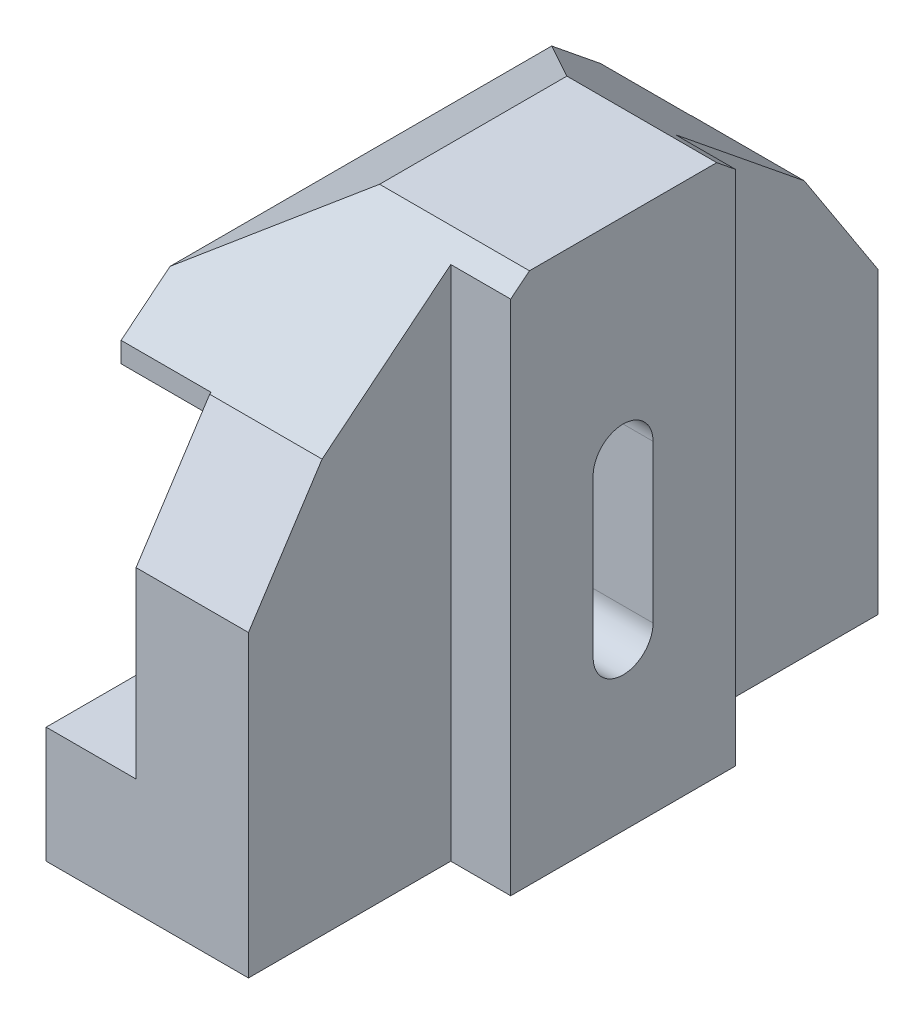
ISO-10303-21;
HEADER;
FILE_DESCRIPTION(('STEP AP214'),'2;1');
FILE_NAME('part.step','',(''),(''),'','','');
FILE_SCHEMA(('AUTOMOTIVE_DESIGN { 1 0 10303 214 1 1 1 1 }'));
ENDSEC;
DATA;
#1=APPLICATION_CONTEXT('core data for automotive mechanical design processes');
#2=APPLICATION_PROTOCOL_DEFINITION('international standard','automotive_design',2000,#1);
#3=PRODUCT_CONTEXT('',#1,'mechanical');
#4=PRODUCT('Part','Part','',(#3));
#5=PRODUCT_RELATED_PRODUCT_CATEGORY('part','',(#4));
#6=PRODUCT_DEFINITION_FORMATION('','',#4);
#7=PRODUCT_DEFINITION_CONTEXT('part definition',#1,'design');
#8=PRODUCT_DEFINITION('design','',#6,#7);
#9=PRODUCT_DEFINITION_SHAPE('','',#8);
#10=(LENGTH_UNIT() NAMED_UNIT(*) SI_UNIT(.MILLI.,.METRE.));
#11=(NAMED_UNIT(*) PLANE_ANGLE_UNIT() SI_UNIT($,.RADIAN.));
#12=(NAMED_UNIT(*) SI_UNIT($,.STERADIAN.) SOLID_ANGLE_UNIT());
#13=UNCERTAINTY_MEASURE_WITH_UNIT(LENGTH_MEASURE(1.E-05),#10,'distance_accuracy_value','');
#14=(GEOMETRIC_REPRESENTATION_CONTEXT(3) GLOBAL_UNCERTAINTY_ASSIGNED_CONTEXT((#13)) GLOBAL_UNIT_ASSIGNED_CONTEXT((#10,
#11,#12)) REPRESENTATION_CONTEXT('',''));
#15=CARTESIAN_POINT('',(0.,0.,0.));
#16=DIRECTION('',(0.,0.,1.));
#17=DIRECTION('',(1.,0.,0.));
#18=AXIS2_PLACEMENT_3D('',#15,#16,#17);
#19=CARTESIAN_POINT('',(27.,0.,84.));
#20=DIRECTION('',(-1.,0.,0.));
#21=DIRECTION('',(0.,0.,1.));
#22=AXIS2_PLACEMENT_3D('',#19,#20,#21);
#23=PLANE('',#22);
#24=DIRECTION('',(0.,-1.,0.));
#25=VECTOR('',#24,1.);
#26=CARTESIAN_POINT('',(27.,71.,57.));
#27=LINE('',#26,#25);
#28=CARTESIAN_POINT('',(27.,68.9755399170125,57.));
#29=VERTEX_POINT('',#28);
#30=CARTESIAN_POINT('',(27.,0.,57.));
#31=VERTEX_POINT('',#30);
#32=EDGE_CURVE('E276',#29,#31,#27,.T.);
#33=ORIENTED_EDGE('',*,*,#32,.F.);
#34=DIRECTION('',(0.,-0.629320391049835,0.777145961456973));
#35=VECTOR('',#34,1.);
#36=CARTESIAN_POINT('',(27.,28.453187913207,107.040937265612));
#37=LINE('',#36,#35);
#38=CARTESIAN_POINT('',(27.,55.0670132063228,74.1756000866226));
#39=VERTEX_POINT('',#38);
#40=EDGE_CURVE('E259',#29,#39,#37,.T.);
#41=ORIENTED_EDGE('',*,*,#40,.T.);
#42=DIRECTION('',(0.,-0.838670567945423,0.544639035015028));
#43=VECTOR('',#42,1.);
#44=CARTESIAN_POINT('',(27.,11.8471025978211,102.242938213101));
#45=LINE('',#44,#43);
#46=CARTESIAN_POINT('',(27.,39.93876398921,84.));
#47=VERTEX_POINT('',#46);
#48=EDGE_CURVE('E275',#39,#47,#45,.T.);
#49=ORIENTED_EDGE('',*,*,#48,.T.);
#50=DIRECTION('',(0.,1.,0.));
#51=VECTOR('',#50,1.);
#52=CARTESIAN_POINT('',(27.,0.,84.));
#53=LINE('',#52,#51);
#54=CARTESIAN_POINT('',(27.,0.,84.));
#55=VERTEX_POINT('',#54);
#56=EDGE_CURVE('E316',#55,#47,#53,.T.);
#57=ORIENTED_EDGE('',*,*,#56,.F.);
#58=DIRECTION('',(0.,0.,-1.));
#59=VECTOR('',#58,1.);
#60=CARTESIAN_POINT('',(27.,0.,84.));
#61=LINE('',#60,#59);
#62=EDGE_CURVE('E358',#55,#31,#61,.T.);
#63=ORIENTED_EDGE('',*,*,#62,.T.);
#64=EDGE_LOOP('',(#33,#41,#49,#57,#63));
#65=FACE_BOUND('',#64,.T.);
#66=ADVANCED_FACE('F39',(#65),#23,.F.);
#67=CARTESIAN_POINT('',(15.,71.,84.));
#68=DIRECTION('',(0.573576436351045,-0.819152044288992,0.));
#69=DIRECTION('',(0.819152044288992,0.573576436351045,0.));
#70=AXIS2_PLACEMENT_3D('',#67,#68,#69);
#71=PLANE('',#70);
#72=DIRECTION('',(0.,0.,-1.));
#73=VECTOR('',#72,1.);
#74=CARTESIAN_POINT('',(15.,71.,84.));
#75=LINE('',#74,#73);
#76=CARTESIAN_POINT('',(15.,71.,54.5));
#77=VERTEX_POINT('',#76);
#78=CARTESIAN_POINT('',(15.,71.,29.5));
#79=VERTEX_POINT('',#78);
#80=EDGE_CURVE('E354',#77,#79,#75,.T.);
#81=ORIENTED_EDGE('',*,*,#80,.T.);
#82=DIRECTION('',(-0.66845613754,-0.468058026468054,-0.578003525978809));
#83=VECTOR('',#82,1.);
#84=CARTESIAN_POINT('',(36.0571652430861,85.7443858365364,47.7078001443945));
#85=LINE('',#84,#83);
#86=CARTESIAN_POINT('',(0.,60.4968869268544,16.5297355312063));
#87=VERTEX_POINT('',#86);
#88=EDGE_CURVE('E255',#79,#87,#85,.T.);
#89=ORIENTED_EDGE('',*,*,#88,.T.);
#90=DIRECTION('',(0.,0.,-1.));
#91=VECTOR('',#90,1.);
#92=CARTESIAN_POINT('',(0.,60.4968869268544,84.));
#93=LINE('',#92,#91);
#94=CARTESIAN_POINT('',(0.,60.4968869268544,67.4702644687937));
#95=VERTEX_POINT('',#94);
#96=EDGE_CURVE('E348',#95,#87,#93,.T.);
#97=ORIENTED_EDGE('',*,*,#96,.F.);
#98=DIRECTION('',(0.668456137539999,0.468058026468053,-0.57800352597881));
#99=VECTOR('',#98,1.);
#100=CARTESIAN_POINT('',(3.60208486842126,63.0190939049941,64.3555982432961));
#101=LINE('',#100,#99);
#102=EDGE_CURVE('E266',#95,#77,#101,.T.);
#103=ORIENTED_EDGE('',*,*,#102,.T.);
#104=EDGE_LOOP('',(#81,#89,#97,#103));
#105=FACE_BOUND('',#104,.T.);
#106=ADVANCED_FACE('F400',(#105),#71,.F.);
#107=CARTESIAN_POINT('',(0.,60.4968869268544,84.));
#108=DIRECTION('',(1.,0.,0.));
#109=DIRECTION('',(0.,1.,0.));
#110=AXIS2_PLACEMENT_3D('',#107,#108,#109);
#111=PLANE('',#110);
#112=ORIENTED_EDGE('',*,*,#96,.T.);
#113=DIRECTION('',(0.,-0.629320391049836,-0.777145961456972));
#114=VECTOR('',#113,1.);
#115=CARTESIAN_POINT('',(0.,93.4948255823673,57.2787961484174));
#116=LINE('',#115,#114);
#117=CARTESIAN_POINT('',(0.,55.2092113526974,10.));
#118=VERTEX_POINT('',#117);
#119=EDGE_CURVE('E248',#87,#118,#116,.T.);
#120=ORIENTED_EDGE('',*,*,#119,.T.);
#121=DIRECTION('',(0.,-1.,0.));
#122=VECTOR('',#121,1.);
#123=CARTESIAN_POINT('',(0.,99.4968869268544,10.));
#124=LINE('',#123,#122);
#125=CARTESIAN_POINT('',(0.,52.4968869268544,10.));
#126=VERTEX_POINT('',#125);
#127=EDGE_CURVE('E296',#118,#126,#124,.T.);
#128=ORIENTED_EDGE('',*,*,#127,.T.);
#129=DIRECTION('',(0.,0.,-1.));
#130=VECTOR('',#129,1.);
#131=CARTESIAN_POINT('',(0.,52.4968869268544,84.));
#132=LINE('',#131,#130);
#133=CARTESIAN_POINT('',(0.,52.4968869268544,74.));
#134=VERTEX_POINT('',#133);
#135=EDGE_CURVE('E349',#134,#126,#132,.T.);
#136=ORIENTED_EDGE('',*,*,#135,.F.);
#137=DIRECTION('',(0.,-1.,0.));
#138=VECTOR('',#137,1.);
#139=CARTESIAN_POINT('',(0.,99.4968869268544,74.));
#140=LINE('',#139,#138);
#141=CARTESIAN_POINT('',(0.,55.2092113526974,74.));
#142=VERTEX_POINT('',#141);
#143=EDGE_CURVE('E299',#142,#134,#140,.T.);
#144=ORIENTED_EDGE('',*,*,#143,.F.);
#145=DIRECTION('',(0.,0.629320391049835,-0.777145961456973));
#146=VECTOR('',#145,1.);
#147=CARTESIAN_POINT('',(0.,52.4126263515475,77.4534948659287));
#148=LINE('',#147,#146);
#149=EDGE_CURVE('E267',#142,#95,#148,.T.);
#150=ORIENTED_EDGE('',*,*,#149,.T.);
#151=EDGE_LOOP('',(#112,#120,#128,#136,#144,#150));
#152=FACE_BOUND('',#151,.T.);
#153=ADVANCED_FACE('F407',(#152),#111,.F.);
#154=CARTESIAN_POINT('',(0.,52.4968869268544,84.));
#155=DIRECTION('',(0.,1.,0.));
#156=DIRECTION('',(0.,0.,1.));
#157=AXIS2_PLACEMENT_3D('',#154,#155,#156);
#158=PLANE('',#157);
#159=DIRECTION('',(1.,0.,0.));
#160=VECTOR('',#159,1.);
#161=CARTESIAN_POINT('',(0.,52.4968869268544,74.));
#162=LINE('',#161,#160);
#163=CARTESIAN_POINT('',(12.,52.4968869268544,74.));
#164=VERTEX_POINT('',#163);
#165=EDGE_CURVE('E307',#134,#164,#162,.T.);
#166=ORIENTED_EDGE('',*,*,#165,.F.);
#167=ORIENTED_EDGE('',*,*,#135,.T.);
#168=DIRECTION('',(-1.,0.,0.));
#169=VECTOR('',#168,1.);
#170=CARTESIAN_POINT('',(0.,52.4968869268544,10.));
#171=LINE('',#170,#169);
#172=CARTESIAN_POINT('',(12.,52.4968869268544,10.));
#173=VERTEX_POINT('',#172);
#174=EDGE_CURVE('E302',#173,#126,#171,.T.);
#175=ORIENTED_EDGE('',*,*,#174,.F.);
#176=DIRECTION('',(0.,0.,-1.));
#177=VECTOR('',#176,1.);
#178=CARTESIAN_POINT('',(12.,52.4968869268544,84.));
#179=LINE('',#178,#177);
#180=EDGE_CURVE('E344',#164,#173,#179,.T.);
#181=ORIENTED_EDGE('',*,*,#180,.F.);
#182=EDGE_LOOP('',(#166,#167,#175,#181));
#183=FACE_BOUND('',#182,.T.);
#184=ADVANCED_FACE('F477',(#183),#158,.F.);
#185=CARTESIAN_POINT('',(0.,0.,84.));
#186=DIRECTION('',(0.,0.,1.));
#187=DIRECTION('',(1.,0.,0.));
#188=AXIS2_PLACEMENT_3D('',#185,#186,#187);
#189=PLANE('',#188);
#190=DIRECTION('',(1.,0.,0.));
#191=VECTOR('',#190,1.);
#192=CARTESIAN_POINT('',(-15.5,39.93876398921,84.));
#193=LINE('',#192,#191);
#194=CARTESIAN_POINT('',(12.,39.93876398921,84.));
#195=VERTEX_POINT('',#194);
#196=EDGE_CURVE('E235',#195,#47,#193,.T.);
#197=ORIENTED_EDGE('',*,*,#196,.F.);
#198=DIRECTION('',(0.,-1.,0.));
#199=VECTOR('',#198,1.);
#200=CARTESIAN_POINT('',(12.,52.4968869268544,84.));
#201=LINE('',#200,#199);
#202=CARTESIAN_POINT('',(12.,15.4968869268544,84.));
#203=VERTEX_POINT('',#202);
#204=EDGE_CURVE('E325',#195,#203,#201,.T.);
#205=ORIENTED_EDGE('',*,*,#204,.T.);
#206=DIRECTION('',(-1.,0.,0.));
#207=VECTOR('',#206,1.);
#208=CARTESIAN_POINT('',(12.,15.4968869268544,84.));
#209=LINE('',#208,#207);
#210=CARTESIAN_POINT('',(0.,15.4968869268544,84.));
#211=VERTEX_POINT('',#210);
#212=EDGE_CURVE('E321',#203,#211,#209,.T.);
#213=ORIENTED_EDGE('',*,*,#212,.T.);
#214=DIRECTION('',(0.,-1.,0.));
#215=VECTOR('',#214,1.);
#216=CARTESIAN_POINT('',(0.,15.4968869268544,84.));
#217=LINE('',#216,#215);
#218=CARTESIAN_POINT('',(0.,0.,84.));
#219=VERTEX_POINT('',#218);
#220=EDGE_CURVE('E312',#211,#219,#217,.T.);
#221=ORIENTED_EDGE('',*,*,#220,.T.);
#222=DIRECTION('',(1.,0.,0.));
#223=VECTOR('',#222,1.);
#224=CARTESIAN_POINT('',(0.,0.,84.));
#225=LINE('',#224,#223);
#226=EDGE_CURVE('E317',#219,#55,#225,.T.);
#227=ORIENTED_EDGE('',*,*,#226,.T.);
#228=ORIENTED_EDGE('',*,*,#56,.T.);
#229=EDGE_LOOP('',(#197,#205,#213,#221,#227,#228));
#230=FACE_BOUND('',#229,.T.);
#231=ADVANCED_FACE('F463',(#230),#189,.T.);
#232=CARTESIAN_POINT('',(0.,0.,0.));
#233=DIRECTION('',(0.,0.,1.));
#234=DIRECTION('',(1.,0.,0.));
#235=AXIS2_PLACEMENT_3D('',#232,#233,#234);
#236=PLANE('',#235);
#237=DIRECTION('',(0.,-1.,0.));
#238=VECTOR('',#237,1.);
#239=CARTESIAN_POINT('',(12.,52.4968869268544,0.));
#240=LINE('',#239,#238);
#241=CARTESIAN_POINT('',(12.,39.93876398921,0.));
#242=VERTEX_POINT('',#241);
#243=CARTESIAN_POINT('',(12.,15.4968869268544,0.));
#244=VERTEX_POINT('',#243);
#245=EDGE_CURVE('E333',#242,#244,#240,.T.);
#246=ORIENTED_EDGE('',*,*,#245,.F.);
#247=DIRECTION('',(1.,0.,0.));
#248=VECTOR('',#247,1.);
#249=CARTESIAN_POINT('',(-15.5,39.93876398921,0.));
#250=LINE('',#249,#248);
#251=CARTESIAN_POINT('',(27.,39.93876398921,0.));
#252=VERTEX_POINT('',#251);
#253=EDGE_CURVE('E225',#242,#252,#250,.T.);
#254=ORIENTED_EDGE('',*,*,#253,.T.);
#255=DIRECTION('',(0.,1.,0.));
#256=VECTOR('',#255,1.);
#257=CARTESIAN_POINT('',(27.,0.,0.));
#258=LINE('',#257,#256);
#259=CARTESIAN_POINT('',(27.,0.,0.));
#260=VERTEX_POINT('',#259);
#261=EDGE_CURVE('E334',#260,#252,#258,.T.);
#262=ORIENTED_EDGE('',*,*,#261,.F.);
#263=DIRECTION('',(1.,0.,0.));
#264=VECTOR('',#263,1.);
#265=CARTESIAN_POINT('',(0.,0.,0.));
#266=LINE('',#265,#264);
#267=CARTESIAN_POINT('',(0.,0.,0.));
#268=VERTEX_POINT('',#267);
#269=EDGE_CURVE('E328',#268,#260,#266,.T.);
#270=ORIENTED_EDGE('',*,*,#269,.F.);
#271=DIRECTION('',(0.,-1.,0.));
#272=VECTOR('',#271,1.);
#273=CARTESIAN_POINT('',(0.,15.4968869268544,0.));
#274=LINE('',#273,#272);
#275=CARTESIAN_POINT('',(0.,15.4968869268544,0.));
#276=VERTEX_POINT('',#275);
#277=EDGE_CURVE('E315',#276,#268,#274,.T.);
#278=ORIENTED_EDGE('',*,*,#277,.F.);
#279=DIRECTION('',(-1.,0.,0.));
#280=VECTOR('',#279,1.);
#281=CARTESIAN_POINT('',(12.,15.4968869268544,0.));
#282=LINE('',#281,#280);
#283=EDGE_CURVE('E320',#244,#276,#282,.T.);
#284=ORIENTED_EDGE('',*,*,#283,.F.);
#285=EDGE_LOOP('',(#246,#254,#262,#270,#278,#284));
#286=FACE_BOUND('',#285,.T.);
#287=ADVANCED_FACE('F424',(#286),#236,.F.);
#288=CARTESIAN_POINT('',(0.,15.4968869268544,84.));
#289=DIRECTION('',(1.,0.,0.));
#290=DIRECTION('',(0.,1.,0.));
#291=AXIS2_PLACEMENT_3D('',#288,#289,#290);
#292=PLANE('',#291);
#293=ORIENTED_EDGE('',*,*,#277,.T.);
#294=DIRECTION('',(0.,0.,-1.));
#295=VECTOR('',#294,1.);
#296=CARTESIAN_POINT('',(0.,0.,84.));
#297=LINE('',#296,#295);
#298=EDGE_CURVE('E360',#219,#268,#297,.T.);
#299=ORIENTED_EDGE('',*,*,#298,.F.);
#300=ORIENTED_EDGE('',*,*,#220,.F.);
#301=DIRECTION('',(0.,0.,-1.));
#302=VECTOR('',#301,1.);
#303=CARTESIAN_POINT('',(0.,15.4968869268544,84.));
#304=LINE('',#303,#302);
#305=EDGE_CURVE('E329',#211,#276,#304,.T.);
#306=ORIENTED_EDGE('',*,*,#305,.T.);
#307=EDGE_LOOP('',(#293,#299,#300,#306));
#308=FACE_BOUND('',#307,.T.);
#309=ADVANCED_FACE('F41',(#308),#292,.F.);
#310=CARTESIAN_POINT('',(0.,0.,84.));
#311=DIRECTION('',(0.,1.,0.));
#312=DIRECTION('',(0.,0.,1.));
#313=AXIS2_PLACEMENT_3D('',#310,#311,#312);
#314=PLANE('',#313);
#315=ORIENTED_EDGE('',*,*,#269,.T.);
#316=CARTESIAN_POINT('',(27.,0.,27.));
#317=VERTEX_POINT('',#316);
#318=EDGE_CURVE('E353',#317,#260,#61,.T.);
#319=ORIENTED_EDGE('',*,*,#318,.F.);
#320=DIRECTION('',(1.,0.,0.));
#321=VECTOR('',#320,1.);
#322=CARTESIAN_POINT('',(27.,0.,27.));
#323=LINE('',#322,#321);
#324=CARTESIAN_POINT('',(35.,0.,27.));
#325=VERTEX_POINT('',#324);
#326=EDGE_CURVE('E286',#317,#325,#323,.T.);
#327=ORIENTED_EDGE('',*,*,#326,.T.);
#328=DIRECTION('',(0.,0.,-1.));
#329=VECTOR('',#328,1.);
#330=CARTESIAN_POINT('',(35.,0.,57.));
#331=LINE('',#330,#329);
#332=CARTESIAN_POINT('',(35.,0.,57.));
#333=VERTEX_POINT('',#332);
#334=EDGE_CURVE('E294',#333,#325,#331,.T.);
#335=ORIENTED_EDGE('',*,*,#334,.F.);
#336=DIRECTION('',(1.,0.,0.));
#337=VECTOR('',#336,1.);
#338=CARTESIAN_POINT('',(27.,0.,57.));
#339=LINE('',#338,#337);
#340=EDGE_CURVE('E284',#31,#333,#339,.T.);
#341=ORIENTED_EDGE('',*,*,#340,.F.);
#342=ORIENTED_EDGE('',*,*,#62,.F.);
#343=ORIENTED_EDGE('',*,*,#226,.F.);
#344=ORIENTED_EDGE('',*,*,#298,.T.);
#345=EDGE_LOOP('',(#315,#319,#327,#335,#341,#342,#343,#344));
#346=FACE_BOUND('',#345,.T.);
#347=ADVANCED_FACE('F415',(#346),#314,.F.);
#348=ORIENTED_EDGE('',*,*,#261,.T.);
#349=DIRECTION('',(0.,0.838670567945423,0.544639035015029));
#350=VECTOR('',#349,1.);
#351=CARTESIAN_POINT('',(27.,50.2160118188104,6.67412277771519));
#352=LINE('',#351,#350);
#353=CARTESIAN_POINT('',(27.,55.0670132063228,9.82439991337739));
#354=VERTEX_POINT('',#353);
#355=EDGE_CURVE('E273',#252,#354,#352,.T.);
#356=ORIENTED_EDGE('',*,*,#355,.T.);
#357=DIRECTION('',(0.,0.629320391049836,0.777145961456972));
#358=VECTOR('',#357,1.);
#359=CARTESIAN_POINT('',(27.,69.5353871440268,27.691353748734));
#360=LINE('',#359,#358);
#361=CARTESIAN_POINT('',(27.,68.9755399170125,27.));
#362=VERTEX_POINT('',#361);
#363=EDGE_CURVE('E241',#354,#362,#360,.T.);
#364=ORIENTED_EDGE('',*,*,#363,.T.);
#365=DIRECTION('',(0.,-1.,0.));
#366=VECTOR('',#365,1.);
#367=CARTESIAN_POINT('',(27.,71.,27.));
#368=LINE('',#367,#366);
#369=EDGE_CURVE('E279',#362,#317,#368,.T.);
#370=ORIENTED_EDGE('',*,*,#369,.T.);
#371=ORIENTED_EDGE('',*,*,#318,.T.);
#372=EDGE_LOOP('',(#348,#356,#364,#370,#371));
#373=FACE_BOUND('',#372,.T.);
#374=ADVANCED_FACE('F402',(#373),#23,.F.);
#375=CARTESIAN_POINT('',(27.,71.,84.));
#376=DIRECTION('',(0.,-1.,0.));
#377=DIRECTION('',(0.,0.,-1.));
#378=AXIS2_PLACEMENT_3D('',#375,#376,#377);
#379=PLANE('',#378);
#380=DIRECTION('',(0.,0.,-1.));
#381=VECTOR('',#380,1.);
#382=CARTESIAN_POINT('',(35.,71.,57.));
#383=LINE('',#382,#381);
#384=CARTESIAN_POINT('',(35.,71.,54.5));
#385=VERTEX_POINT('',#384);
#386=CARTESIAN_POINT('',(35.,71.,29.5));
#387=VERTEX_POINT('',#386);
#388=EDGE_CURVE('E289',#385,#387,#383,.T.);
#389=ORIENTED_EDGE('',*,*,#388,.T.);
#390=DIRECTION('',(1.,0.,0.));
#391=VECTOR('',#390,1.);
#392=CARTESIAN_POINT('',(-15.5,71.,29.5));
#393=LINE('',#392,#391);
#394=EDGE_CURVE('E229',#79,#387,#393,.T.);
#395=ORIENTED_EDGE('',*,*,#394,.F.);
#396=ORIENTED_EDGE('',*,*,#80,.F.);
#397=DIRECTION('',(1.,0.,0.));
#398=VECTOR('',#397,1.);
#399=CARTESIAN_POINT('',(-15.5,71.,54.5));
#400=LINE('',#399,#398);
#401=EDGE_CURVE('E217',#77,#385,#400,.T.);
#402=ORIENTED_EDGE('',*,*,#401,.T.);
#403=EDGE_LOOP('',(#389,#395,#396,#402));
#404=FACE_BOUND('',#403,.T.);
#405=ADVANCED_FACE('F411',(#404),#379,.F.);
#406=CARTESIAN_POINT('',(12.,52.4968869268544,84.));
#407=DIRECTION('',(1.,0.,0.));
#408=DIRECTION('',(0.,1.,0.));
#409=AXIS2_PLACEMENT_3D('',#406,#407,#408);
#410=PLANE('',#409);
#411=DIRECTION('',(0.,-1.,0.));
#412=VECTOR('',#411,1.);
#413=CARTESIAN_POINT('',(12.,43.0355530867048,38.));
#414=LINE('',#413,#412);
#415=CARTESIAN_POINT('',(12.,43.0355530867048,38.));
#416=VERTEX_POINT('',#415);
#417=CARTESIAN_POINT('',(12.,22.0355530867048,38.));
#418=VERTEX_POINT('',#417);
#419=EDGE_CURVE('E207',#416,#418,#414,.T.);
#420=ORIENTED_EDGE('',*,*,#419,.F.);
#421=CARTESIAN_POINT('',(12.,43.0355530867048,42.));
#422=DIRECTION('',(-1.,0.,0.));
#423=DIRECTION('',(0.,-1.,0.));
#424=AXIS2_PLACEMENT_3D('',#421,#422,#423);
#425=CIRCLE('',#424,4.);
#426=CARTESIAN_POINT('',(12.,43.0355530867048,46.));
#427=VERTEX_POINT('',#426);
#428=EDGE_CURVE('E53',#427,#416,#425,.T.);
#429=ORIENTED_EDGE('',*,*,#428,.F.);
#430=DIRECTION('',(0.,1.,0.));
#431=VECTOR('',#430,1.);
#432=CARTESIAN_POINT('',(12.,43.0355530867048,46.));
#433=LINE('',#432,#431);
#434=CARTESIAN_POINT('',(12.,22.0355530867048,46.));
#435=VERTEX_POINT('',#434);
#436=EDGE_CURVE('E214',#435,#427,#433,.T.);
#437=ORIENTED_EDGE('',*,*,#436,.F.);
#438=CARTESIAN_POINT('',(12.,22.0355530867048,42.));
#439=DIRECTION('',(-1.,0.,0.));
#440=DIRECTION('',(0.,-1.,0.));
#441=AXIS2_PLACEMENT_3D('',#438,#439,#440);
#442=CIRCLE('',#441,3.99999999999999);
#443=EDGE_CURVE('E196',#418,#435,#442,.T.);
#444=ORIENTED_EDGE('',*,*,#443,.F.);
#445=EDGE_LOOP('',(#420,#429,#437,#444));
#446=FACE_BOUND('',#445,.T.);
#447=DIRECTION('',(0.,-0.629320391049836,-0.777145961456972));
#448=VECTOR('',#447,1.);
#449=CARTESIAN_POINT('',(12.,90.3264723456383,53.3662057454822));
#450=LINE('',#449,#448);
#451=CARTESIAN_POINT('',(12.,55.2092113526974,10.));
#452=VERTEX_POINT('',#451);
#453=CARTESIAN_POINT('',(12.,55.0670132063228,9.82439991337739));
#454=VERTEX_POINT('',#453);
#455=EDGE_CURVE('E246',#452,#454,#450,.T.);
#456=ORIENTED_EDGE('',*,*,#455,.T.);
#457=DIRECTION('',(0.,-0.838670567945423,-0.544639035015029));
#458=VECTOR('',#457,1.);
#459=CARTESIAN_POINT('',(12.,87.1406590625168,30.6532690739178));
#460=LINE('',#459,#458);
#461=EDGE_CURVE('E369',#454,#242,#460,.T.);
#462=ORIENTED_EDGE('',*,*,#461,.T.);
#463=ORIENTED_EDGE('',*,*,#245,.T.);
#464=DIRECTION('',(0.,0.,-1.));
#465=VECTOR('',#464,1.);
#466=CARTESIAN_POINT('',(12.,15.4968869268544,84.));
#467=LINE('',#466,#465);
#468=EDGE_CURVE('E338',#203,#244,#467,.T.);
#469=ORIENTED_EDGE('',*,*,#468,.F.);
#470=ORIENTED_EDGE('',*,*,#204,.F.);
#471=DIRECTION('',(0.,0.838670567945423,-0.544639035015028));
#472=VECTOR('',#471,1.);
#473=CARTESIAN_POINT('',(12.,48.7717498415275,78.2637919168988));
#474=LINE('',#473,#472);
#475=CARTESIAN_POINT('',(12.,55.0670132063228,74.1756000866226));
#476=VERTEX_POINT('',#475);
#477=EDGE_CURVE('E370',#195,#476,#474,.T.);
#478=ORIENTED_EDGE('',*,*,#477,.T.);
#479=DIRECTION('',(0.,0.629320391049835,-0.777145961456973));
#480=VECTOR('',#479,1.);
#481=CARTESIAN_POINT('',(12.,49.2442731148185,81.3660852688639));
#482=LINE('',#481,#480);
#483=CARTESIAN_POINT('',(12.,55.2092113526974,74.));
#484=VERTEX_POINT('',#483);
#485=EDGE_CURVE('E265',#476,#484,#482,.T.);
#486=ORIENTED_EDGE('',*,*,#485,.T.);
#487=DIRECTION('',(0.,-1.,0.));
#488=VECTOR('',#487,1.);
#489=CARTESIAN_POINT('',(12.,99.4968869268544,74.));
#490=LINE('',#489,#488);
#491=EDGE_CURVE('E301',#484,#164,#490,.T.);
#492=ORIENTED_EDGE('',*,*,#491,.T.);
#493=ORIENTED_EDGE('',*,*,#180,.T.);
#494=DIRECTION('',(0.,-1.,0.));
#495=VECTOR('',#494,1.);
#496=CARTESIAN_POINT('',(12.,99.4968869268544,10.));
#497=LINE('',#496,#495);
#498=EDGE_CURVE('E305',#452,#173,#497,.T.);
#499=ORIENTED_EDGE('',*,*,#498,.F.);
#500=EDGE_LOOP('',(#456,#462,#463,#469,#470,#478,#486,#492,#493,#499));
#501=FACE_BOUND('',#500,.T.);
#502=ADVANCED_FACE('F208',(#446,#501),#410,.F.);
#503=CARTESIAN_POINT('',(12.,15.4968869268544,84.));
#504=DIRECTION('',(0.,-1.,0.));
#505=DIRECTION('',(1.,0.,0.));
#506=AXIS2_PLACEMENT_3D('',#503,#504,#505);
#507=PLANE('',#506);
#508=ORIENTED_EDGE('',*,*,#283,.T.);
#509=ORIENTED_EDGE('',*,*,#305,.F.);
#510=ORIENTED_EDGE('',*,*,#212,.F.);
#511=ORIENTED_EDGE('',*,*,#468,.T.);
#512=EDGE_LOOP('',(#508,#509,#510,#511));
#513=FACE_BOUND('',#512,.T.);
#514=ADVANCED_FACE('F457',(#513),#507,.F.);
#515=CARTESIAN_POINT('',(0.,99.4968869268544,10.));
#516=DIRECTION('',(0.,0.,-1.));
#517=DIRECTION('',(-1.,0.,0.));
#518=AXIS2_PLACEMENT_3D('',#515,#516,#517);
#519=PLANE('',#518);
#520=DIRECTION('',(-1.,0.,0.));
#521=VECTOR('',#520,1.);
#522=CARTESIAN_POINT('',(0.,55.2092113526974,10.));
#523=LINE('',#522,#521);
#524=EDGE_CURVE('E242',#452,#118,#523,.T.);
#525=ORIENTED_EDGE('',*,*,#524,.F.);
#526=ORIENTED_EDGE('',*,*,#498,.T.);
#527=ORIENTED_EDGE('',*,*,#174,.T.);
#528=ORIENTED_EDGE('',*,*,#127,.F.);
#529=EDGE_LOOP('',(#525,#526,#527,#528));
#530=FACE_BOUND('',#529,.T.);
#531=ADVANCED_FACE('F438',(#530),#519,.T.);
#532=CARTESIAN_POINT('',(0.,99.4968869268544,74.));
#533=DIRECTION('',(0.,0.,1.));
#534=DIRECTION('',(1.,0.,0.));
#535=AXIS2_PLACEMENT_3D('',#532,#533,#534);
#536=PLANE('',#535);
#537=DIRECTION('',(1.,0.,0.));
#538=VECTOR('',#537,1.);
#539=CARTESIAN_POINT('',(0.,55.2092113526974,74.));
#540=LINE('',#539,#538);
#541=EDGE_CURVE('E264',#142,#484,#540,.T.);
#542=ORIENTED_EDGE('',*,*,#541,.F.);
#543=ORIENTED_EDGE('',*,*,#143,.T.);
#544=ORIENTED_EDGE('',*,*,#165,.T.);
#545=ORIENTED_EDGE('',*,*,#491,.F.);
#546=EDGE_LOOP('',(#542,#543,#544,#545));
#547=FACE_BOUND('',#546,.T.);
#548=ADVANCED_FACE('F479',(#547),#536,.T.);
#549=CARTESIAN_POINT('',(35.,71.,57.));
#550=DIRECTION('',(-1.,0.,0.));
#551=DIRECTION('',(0.,-1.,0.));
#552=AXIS2_PLACEMENT_3D('',#549,#550,#551);
#553=PLANE('',#552);
#554=DIRECTION('',(0.,1.,0.));
#555=VECTOR('',#554,1.);
#556=CARTESIAN_POINT('',(35.,71.,46.));
#557=LINE('',#556,#555);
#558=CARTESIAN_POINT('',(35.,22.0355530867048,46.));
#559=VERTEX_POINT('',#558);
#560=CARTESIAN_POINT('',(35.,43.0355530867048,46.));
#561=VERTEX_POINT('',#560);
#562=EDGE_CURVE('E50',#559,#561,#557,.T.);
#563=ORIENTED_EDGE('',*,*,#562,.T.);
#564=CARTESIAN_POINT('',(35.,43.0355530867048,42.));
#565=DIRECTION('',(-1.,0.,0.));
#566=DIRECTION('',(0.,-1.,0.));
#567=AXIS2_PLACEMENT_3D('',#564,#565,#566);
#568=CIRCLE('',#567,4.);
#569=CARTESIAN_POINT('',(35.,43.0355530867048,38.));
#570=VERTEX_POINT('',#569);
#571=EDGE_CURVE('E11',#561,#570,#568,.T.);
#572=ORIENTED_EDGE('',*,*,#571,.T.);
#573=DIRECTION('',(0.,-1.,0.));
#574=VECTOR('',#573,1.);
#575=CARTESIAN_POINT('',(35.,71.,38.));
#576=LINE('',#575,#574);
#577=CARTESIAN_POINT('',(35.,22.0355530867048,38.));
#578=VERTEX_POINT('',#577);
#579=EDGE_CURVE('E373',#570,#578,#576,.T.);
#580=ORIENTED_EDGE('',*,*,#579,.T.);
#581=CARTESIAN_POINT('',(35.,22.0355530867048,42.));
#582=DIRECTION('',(-1.,0.,0.));
#583=DIRECTION('',(0.,-1.,0.));
#584=AXIS2_PLACEMENT_3D('',#581,#582,#583);
#585=CIRCLE('',#584,3.99999999999999);
#586=EDGE_CURVE('E197',#578,#559,#585,.T.);
#587=ORIENTED_EDGE('',*,*,#586,.T.);
#588=EDGE_LOOP('',(#563,#572,#580,#587));
#589=FACE_BOUND('',#588,.T.);
#590=DIRECTION('',(0.,1.,0.));
#591=VECTOR('',#590,1.);
#592=CARTESIAN_POINT('',(35.,71.,27.));
#593=LINE('',#592,#591);
#594=CARTESIAN_POINT('',(35.,68.9755399170125,27.));
#595=VERTEX_POINT('',#594);
#596=EDGE_CURVE('E281',#325,#595,#593,.T.);
#597=ORIENTED_EDGE('',*,*,#596,.T.);
#598=DIRECTION('',(0.,0.629320391049836,0.777145961456972));
#599=VECTOR('',#598,1.);
#600=CARTESIAN_POINT('',(35.,84.4495295100898,46.1087857487442));
#601=LINE('',#600,#599);
#602=EDGE_CURVE('E228',#595,#387,#601,.T.);
#603=ORIENTED_EDGE('',*,*,#602,.T.);
#604=ORIENTED_EDGE('',*,*,#388,.F.);
#605=DIRECTION('',(0.,-0.629320391049835,0.777145961456973));
#606=VECTOR('',#605,1.);
#607=CARTESIAN_POINT('',(35.,69.7773154990827,56.0098896135222));
#608=LINE('',#607,#606);
#609=CARTESIAN_POINT('',(35.,68.9755399170125,57.));
#610=VERTEX_POINT('',#609);
#611=EDGE_CURVE('E253',#385,#610,#608,.T.);
#612=ORIENTED_EDGE('',*,*,#611,.T.);
#613=DIRECTION('',(0.,1.,0.));
#614=VECTOR('',#613,1.);
#615=CARTESIAN_POINT('',(35.,71.,57.));
#616=LINE('',#615,#614);
#617=EDGE_CURVE('E283',#333,#610,#616,.T.);
#618=ORIENTED_EDGE('',*,*,#617,.F.);
#619=ORIENTED_EDGE('',*,*,#334,.T.);
#620=EDGE_LOOP('',(#597,#603,#604,#612,#618,#619));
#621=FACE_BOUND('',#620,.T.);
#622=ADVANCED_FACE('F380',(#589,#621),#553,.F.);
#623=CARTESIAN_POINT('',(0.,0.,57.));
#624=DIRECTION('',(0.,0.,1.));
#625=DIRECTION('',(1.,0.,0.));
#626=AXIS2_PLACEMENT_3D('',#623,#624,#625);
#627=PLANE('',#626);
#628=DIRECTION('',(1.,0.,0.));
#629=VECTOR('',#628,1.);
#630=CARTESIAN_POINT('',(0.,68.9755399170125,57.));
#631=LINE('',#630,#629);
#632=EDGE_CURVE('E362',#29,#610,#631,.T.);
#633=ORIENTED_EDGE('',*,*,#632,.F.);
#634=ORIENTED_EDGE('',*,*,#32,.T.);
#635=ORIENTED_EDGE('',*,*,#340,.T.);
#636=ORIENTED_EDGE('',*,*,#617,.T.);
#637=EDGE_LOOP('',(#633,#634,#635,#636));
#638=FACE_BOUND('',#637,.T.);
#639=ADVANCED_FACE('F472',(#638),#627,.T.);
#640=CARTESIAN_POINT('',(0.,0.,27.));
#641=DIRECTION('',(0.,0.,1.));
#642=DIRECTION('',(1.,0.,0.));
#643=AXIS2_PLACEMENT_3D('',#640,#641,#642);
#644=PLANE('',#643);
#645=ORIENTED_EDGE('',*,*,#369,.F.);
#646=DIRECTION('',(1.,0.,0.));
#647=VECTOR('',#646,1.);
#648=CARTESIAN_POINT('',(0.,68.9755399170125,27.));
#649=LINE('',#648,#647);
#650=EDGE_CURVE('E365',#362,#595,#649,.T.);
#651=ORIENTED_EDGE('',*,*,#650,.T.);
#652=ORIENTED_EDGE('',*,*,#596,.F.);
#653=ORIENTED_EDGE('',*,*,#326,.F.);
#654=EDGE_LOOP('',(#645,#651,#652,#653));
#655=FACE_BOUND('',#654,.T.);
#656=ADVANCED_FACE('F454',(#655),#644,.F.);
#657=CARTESIAN_POINT('',(-15.5,39.93876398921,0.));
#658=DIRECTION('',(0.,-0.544639035015029,0.838670567945423));
#659=DIRECTION('',(0.,-0.838670567945423,-0.544639035015029));
#660=AXIS2_PLACEMENT_3D('',#657,#658,#659);
#661=PLANE('',#660);
#662=ORIENTED_EDGE('',*,*,#253,.F.);
#663=ORIENTED_EDGE('',*,*,#461,.F.);
#664=DIRECTION('',(1.,0.,0.));
#665=VECTOR('',#664,1.);
#666=CARTESIAN_POINT('',(-15.5,55.0670132063228,9.82439991337739));
#667=LINE('',#666,#665);
#668=EDGE_CURVE('E227',#454,#354,#667,.T.);
#669=ORIENTED_EDGE('',*,*,#668,.T.);
#670=ORIENTED_EDGE('',*,*,#355,.F.);
#671=EDGE_LOOP('',(#662,#663,#669,#670));
#672=FACE_BOUND('',#671,.T.);
#673=ADVANCED_FACE('F429',(#672),#661,.F.);
#674=CARTESIAN_POINT('',(-15.5,71.,29.5));
#675=DIRECTION('',(0.,-0.777145961456972,0.629320391049836));
#676=DIRECTION('',(0.,-0.629320391049836,-0.777145961456972));
#677=AXIS2_PLACEMENT_3D('',#674,#675,#676);
#678=PLANE('',#677);
#679=ORIENTED_EDGE('',*,*,#394,.T.);
#680=ORIENTED_EDGE('',*,*,#602,.F.);
#681=ORIENTED_EDGE('',*,*,#650,.F.);
#682=ORIENTED_EDGE('',*,*,#363,.F.);
#683=ORIENTED_EDGE('',*,*,#668,.F.);
#684=ORIENTED_EDGE('',*,*,#455,.F.);
#685=ORIENTED_EDGE('',*,*,#524,.T.);
#686=ORIENTED_EDGE('',*,*,#119,.F.);
#687=ORIENTED_EDGE('',*,*,#88,.F.);
#688=EDGE_LOOP('',(#679,#680,#681,#682,#683,#684,#685,#686,#687));
#689=FACE_BOUND('',#688,.T.);
#690=ADVANCED_FACE('F434',(#689),#678,.F.);
#691=CARTESIAN_POINT('',(-15.5,39.93876398921,84.));
#692=DIRECTION('',(0.,-0.544639035015028,-0.838670567945423));
#693=DIRECTION('',(0.,0.838670567945423,-0.544639035015028));
#694=AXIS2_PLACEMENT_3D('',#691,#692,#693);
#695=PLANE('',#694);
#696=DIRECTION('',(1.,0.,0.));
#697=VECTOR('',#696,1.);
#698=CARTESIAN_POINT('',(-15.5,55.0670132063228,74.1756000866226));
#699=LINE('',#698,#697);
#700=EDGE_CURVE('E234',#476,#39,#699,.T.);
#701=ORIENTED_EDGE('',*,*,#700,.F.);
#702=ORIENTED_EDGE('',*,*,#477,.F.);
#703=ORIENTED_EDGE('',*,*,#196,.T.);
#704=ORIENTED_EDGE('',*,*,#48,.F.);
#705=EDGE_LOOP('',(#701,#702,#703,#704));
#706=FACE_BOUND('',#705,.T.);
#707=ADVANCED_FACE('F391',(#706),#695,.F.);
#708=CARTESIAN_POINT('',(-15.5,71.,54.5));
#709=DIRECTION('',(0.,-0.777145961456973,-0.629320391049835));
#710=DIRECTION('',(0.,0.629320391049835,-0.777145961456973));
#711=AXIS2_PLACEMENT_3D('',#708,#709,#710);
#712=PLANE('',#711);
#713=ORIENTED_EDGE('',*,*,#149,.F.);
#714=ORIENTED_EDGE('',*,*,#541,.T.);
#715=ORIENTED_EDGE('',*,*,#485,.F.);
#716=ORIENTED_EDGE('',*,*,#700,.T.);
#717=ORIENTED_EDGE('',*,*,#40,.F.);
#718=ORIENTED_EDGE('',*,*,#632,.T.);
#719=ORIENTED_EDGE('',*,*,#611,.F.);
#720=ORIENTED_EDGE('',*,*,#401,.F.);
#721=ORIENTED_EDGE('',*,*,#102,.F.);
#722=EDGE_LOOP('',(#713,#714,#715,#716,#717,#718,#719,#720,#721));
#723=FACE_BOUND('',#722,.T.);
#724=ADVANCED_FACE('F381',(#723),#712,.F.);
#725=CARTESIAN_POINT('',(87.,43.0355530867048,42.));
#726=DIRECTION('',(-1.,0.,0.));
#727=DIRECTION('',(0.,-1.,0.));
#728=AXIS2_PLACEMENT_3D('',#725,#726,#727);
#729=CYLINDRICAL_SURFACE('',#728,4.);
#730=DIRECTION('',(-1.,0.,0.));
#731=VECTOR('',#730,1.);
#732=CARTESIAN_POINT('',(87.,43.0355530867048,46.));
#733=LINE('',#732,#731);
#734=EDGE_CURVE('E220',#561,#427,#733,.T.);
#735=ORIENTED_EDGE('',*,*,#734,.T.);
#736=ORIENTED_EDGE('',*,*,#428,.T.);
#737=DIRECTION('',(-1.,0.,0.));
#738=VECTOR('',#737,1.);
#739=CARTESIAN_POINT('',(87.,43.0355530867048,38.));
#740=LINE('',#739,#738);
#741=EDGE_CURVE('E205',#570,#416,#740,.T.);
#742=ORIENTED_EDGE('',*,*,#741,.F.);
#743=ORIENTED_EDGE('',*,*,#571,.F.);
#744=EDGE_LOOP('',(#735,#736,#742,#743));
#745=FACE_BOUND('',#744,.T.);
#746=ADVANCED_FACE('F385',(#745),#729,.F.);
#747=CARTESIAN_POINT('',(87.,43.0355530867048,46.));
#748=DIRECTION('',(0.,0.,1.));
#749=DIRECTION('',(0.,-1.,0.));
#750=AXIS2_PLACEMENT_3D('',#747,#748,#749);
#751=PLANE('',#750);
#752=DIRECTION('',(-1.,0.,0.));
#753=VECTOR('',#752,1.);
#754=CARTESIAN_POINT('',(87.,22.0355530867048,46.));
#755=LINE('',#754,#753);
#756=EDGE_CURVE('E204',#559,#435,#755,.T.);
#757=ORIENTED_EDGE('',*,*,#756,.T.);
#758=ORIENTED_EDGE('',*,*,#436,.T.);
#759=ORIENTED_EDGE('',*,*,#734,.F.);
#760=ORIENTED_EDGE('',*,*,#562,.F.);
#761=EDGE_LOOP('',(#757,#758,#759,#760));
#762=FACE_BOUND('',#761,.T.);
#763=ADVANCED_FACE('F382',(#762),#751,.F.);
#764=CARTESIAN_POINT('',(87.,22.0355530867048,42.));
#765=DIRECTION('',(-1.,0.,0.));
#766=DIRECTION('',(0.,-1.,0.));
#767=AXIS2_PLACEMENT_3D('',#764,#765,#766);
#768=CYLINDRICAL_SURFACE('',#767,3.99999999999999);
#769=DIRECTION('',(-1.,0.,0.));
#770=VECTOR('',#769,1.);
#771=CARTESIAN_POINT('',(87.,22.0355530867048,38.));
#772=LINE('',#771,#770);
#773=EDGE_CURVE('E65',#578,#418,#772,.T.);
#774=ORIENTED_EDGE('',*,*,#773,.T.);
#775=ORIENTED_EDGE('',*,*,#443,.T.);
#776=ORIENTED_EDGE('',*,*,#756,.F.);
#777=ORIENTED_EDGE('',*,*,#586,.F.);
#778=EDGE_LOOP('',(#774,#775,#776,#777));
#779=FACE_BOUND('',#778,.T.);
#780=ADVANCED_FACE('F191',(#779),#768,.F.);
#781=CARTESIAN_POINT('',(87.,43.0355530867048,38.));
#782=DIRECTION('',(0.,0.,-1.));
#783=DIRECTION('',(0.,1.,0.));
#784=AXIS2_PLACEMENT_3D('',#781,#782,#783);
#785=PLANE('',#784);
#786=ORIENTED_EDGE('',*,*,#741,.T.);
#787=ORIENTED_EDGE('',*,*,#419,.T.);
#788=ORIENTED_EDGE('',*,*,#773,.F.);
#789=ORIENTED_EDGE('',*,*,#579,.F.);
#790=EDGE_LOOP('',(#786,#787,#788,#789));
#791=FACE_BOUND('',#790,.T.);
#792=ADVANCED_FACE('F210',(#791),#785,.F.);
#793=CLOSED_SHELL('',(#66,#106,#153,#184,#231,#287,#309,#347,#374,#405,#502,#514,#531,#548,#622,
#639,#656,#673,#690,#707,#724,#746,#763,#780,#792));
#794=MANIFOLD_SOLID_BREP('B2',#793);
#795=ADVANCED_BREP_SHAPE_REPRESENTATION('',(#18,#794),#14);
#796=SHAPE_DEFINITION_REPRESENTATION(#9,#795);
ENDSEC;
END-ISO-10303-21;
